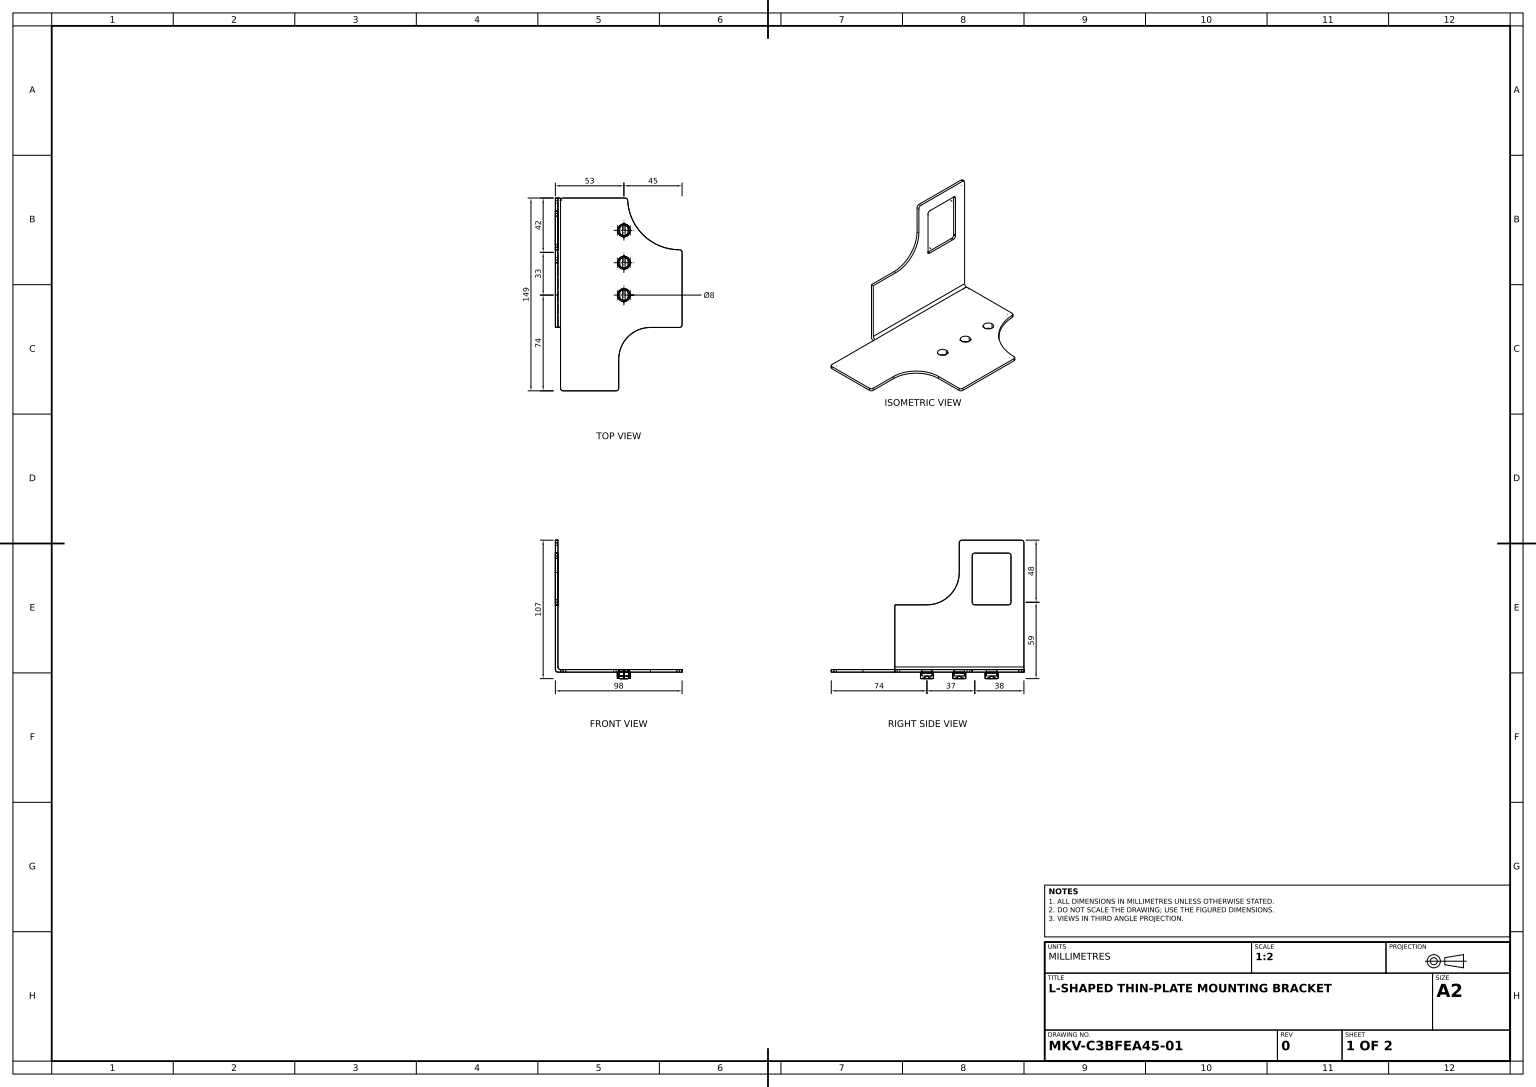
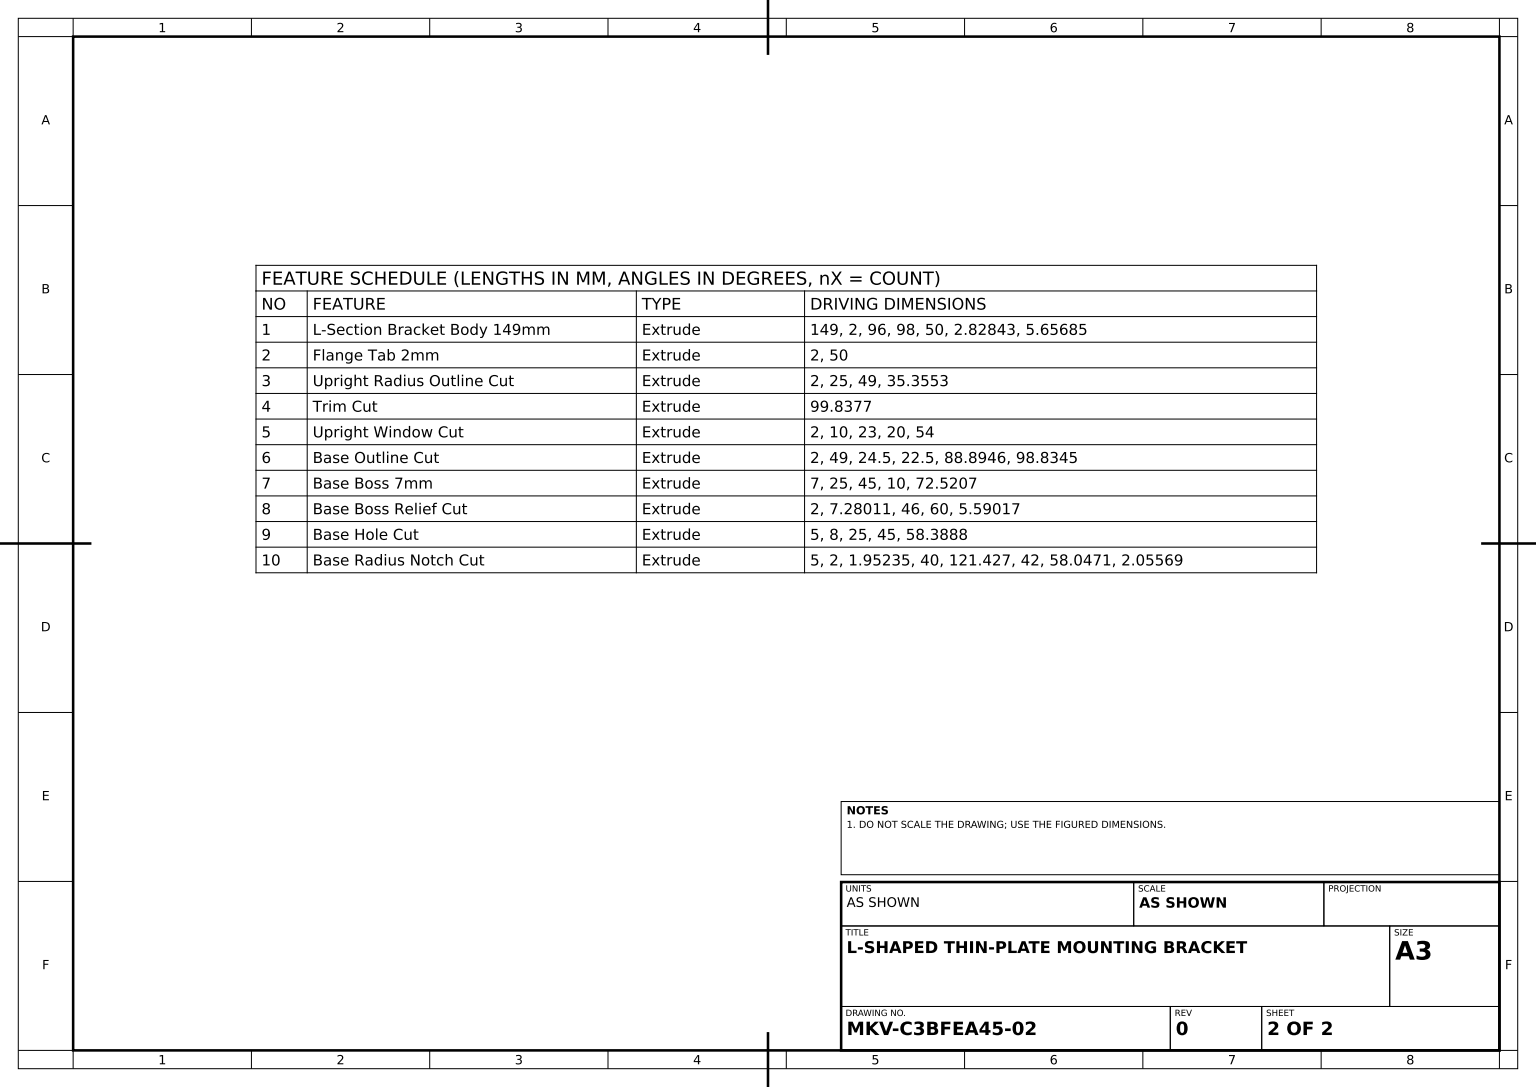
from build123d import *

# Parameters (mm, degrees)
L_SECTION_BRACKET_BODY_149MM_DEPTH = 74.5
FLANGE_TAB_SKETCH_W                = 149
FLANGE_TAB_SKETCH_H                = 50
FLANGE_TAB_2MM_DEPTH               = 2
UPRIGHT_RADIUS_OUTLINE_CUT_DEPTH   = 2
TRIM_CUT_DEPTH                     = 159.600914247
TRIM_CUT_DEPTH_BACK                = 159.600914247
TRIM_CUT_SKETCH_W                  = 4
TRIM_CUT_SKETCH_H                  = 49.162283459
UPRIGHT_WINDOW_CUT_DEPTH           = 2
BASE_OUTLINE_CUT_DEPTH             = 2
BASE_BOSS_SKETCH_R                 = 5
BASE_BOSS_7MM_DEPTH                = 7
BASE_BOSS_RELIEF_CUT_DEPTH         = 160.869478013
BASE_BOSS_RELIEF_CUT_DEPTH_BACK    = 160.869478013
BASE_HOLE_SKETCH_R                 = 4
BASE_HOLE_CUT_DEPTH                = 5
BASE_RADIUS_NOTCH_CUT_DEPTH        = 5


with BuildPart() as part:
    # L-Section Profile Sketch → L-Section Bracket Body 149mm (new, symmetric)
    with BuildSketch(Plane.XY):
        with BuildLine():
            Line((2, 0), (98, 0))
            Line((98, 0), (98, 2))
            Line((98, 2), (4, 2))
            ThreePointArc((4, 2), (2.585786438, 2.585786438), (2, 4))
            Line((2, 4), (2, 52))
            Line((2, 52), (0, 52))
            Line((0, 52), (0, 2))
            ThreePointArc((0, 2), (0.585786438, 0.585786438), (2, 0))
        make_face()
    extrude(amount=L_SECTION_BRACKET_BODY_149MM_DEPTH, both=True)

    # Flange Tab Sketch → Flange Tab 2mm (add)
    with BuildSketch(Plane(origin=(2, 0, 0), x_dir=(0, 0, -1), z_dir=(1, 0, 0))):
        with Locations((0, 77)):
            Rectangle(FLANGE_TAB_SKETCH_W, FLANGE_TAB_SKETCH_H)
    extrude(amount=-FLANGE_TAB_2MM_DEPTH)

    # Upright Radius Outline Sketch → Upright Radius Outline Cut (cut)
    with BuildSketch(Plane(origin=(2, 0, 0), x_dir=(0, 0, -1), z_dir=(1, 0, 0))):
        with BuildLine():
            Line((24.5, 102), (-74.5, 102))
            Line((-74.5, 102), (-74.5, 4))
            Line((-74.5, 4), (-25.5, 4))
            Line((-25.5, 4), (-25.5, 52))
            Line((-25.5, 52), (-0.5, 52))
            ThreePointArc((-0.5, 52), (17.17766953, 59.32233047), (24.5, 77))
            Line((24.5, 77), (24.5, 102))
        make_face()
    extrude(amount=-UPRIGHT_RADIUS_OUTLINE_CUT_DEPTH, mode=Mode.SUBTRACT)

    # Trim Cut Sketch → Trim Cut (cut, two sides: drawn at the far end of the back side and taken through both)
    with BuildSketch(Plane(origin=(0, 2, 0), x_dir=(1, 0, 0), z_dir=(0, 1, 0)).offset(-TRIM_CUT_DEPTH_BACK)):
        with Locations((2, -49.918858271)):
            Rectangle(TRIM_CUT_SKETCH_W, TRIM_CUT_SKETCH_H)
    extrude(amount=TRIM_CUT_DEPTH + TRIM_CUT_DEPTH_BACK, mode=Mode.SUBTRACT)

    # Upright Window Sketch → Upright Window Cut (cut)
    with BuildSketch(Plane(origin=(2, 0, 0), x_dir=(0, 0, -1), z_dir=(1, 0, 0))):
        with BuildLine():
            ThreePointArc((24.5, 100), (25.085786438, 101.414213562), (26.5, 102))
            Line((26.5, 102), (24.5, 102))
            Line((24.5, 102), (24.5, 100))
        make_face()
        with BuildLine():
            Line((74.5, 100), (74.5, 102))
            Line((74.5, 102), (72.5, 102))
            ThreePointArc((72.5, 102), (73.914213562, 101.414213562), (74.5, 100))
        make_face()
        with BuildLine():
            ThreePointArc((36.5, 52), (35.085786438, 52.585786438), (34.5, 54))
            Line((34.5, 54), (34.5, 90))
            ThreePointArc((34.5, 90), (35.085786438, 91.414213562), (36.5, 92))
            Line((36.5, 92), (62.5, 92))
            ThreePointArc((62.5, 92), (63.914213562, 91.414213562), (64.5, 90))
            Line((64.5, 90), (64.5, 54))
            ThreePointArc((64.5, 54), (63.914213562, 52.585786438), (62.5, 52))
            Line((62.5, 52), (36.5, 52))
        make_face()
    extrude(amount=-UPRIGHT_WINDOW_CUT_DEPTH, mode=Mode.SUBTRACT)

    # Base Outline Sketch → Base Outline Cut (cut)
    with BuildSketch(Plane(origin=(0, 2, 0), x_dir=(1, 0, 0), z_dir=(0, 1, 0))):
        with BuildLine():
            Line((6, 74.5), (4, 74.5))
            Line((4, 74.5), (4, 72.5))
            ThreePointArc((4, 72.5), (4.585786438, 73.914213562), (6, 74.5))
        make_face()
        with BuildLine():
            Line((98, -74.5), (98, -23.5))
            ThreePointArc((98, -23.5), (97.414213562, -24.914213562), (96, -25.5))
            Line((96, -25.5), (73.5, -25.5))
            ThreePointArc((73.5, -25.5), (56.175883861, -32.675883861), (49, -50))
            Line((49, -50), (49, -72.5))
            ThreePointArc((49, -72.5), (48.414213562, -73.914213562), (47, -74.5))
            Line((47, -74.5), (98, -74.5))
        make_face()
        with BuildLine():
            ThreePointArc((6, -74.5), (4.585786438, -73.914213562), (4, -72.5))
            Line((4, -72.5), (4, -74.5))
            Line((4, -74.5), (6, -74.5))
        make_face()
    extrude(amount=-BASE_OUTLINE_CUT_DEPTH, mode=Mode.SUBTRACT)

    # Base Boss Sketch → Base Boss 7mm (add)
    with BuildSketch(Plane(origin=(0, 2, 0), x_dir=(1, 0, 0), z_dir=(0, 1, 0))):
        with Locations(Location((53, 24.5, 0), (0, 0, 270))):
            Circle(BASE_BOSS_SKETCH_R)
        with Locations(Location((53, 49.5, 0), (0, 0, 270))):
            Circle(BASE_BOSS_SKETCH_R)
        with Locations(Location((53, -0.5, 0), (0, 0, 270))):
            Circle(BASE_BOSS_SKETCH_R)
    extrude(amount=-BASE_BOSS_7MM_DEPTH)

    # Base Boss Relief Sketch → Base Boss Relief Cut (cut, two sides: drawn at the far end of the back side and taken through both)
    with BuildSketch(Plane.XY.offset(-BASE_BOSS_RELIEF_CUT_DEPTH_BACK)):
        with BuildLine():
            ThreePointArc((48, -3), (48.585786438, -4.414213562), (50, -5))
            Line((50, -5), (48, -5))
            Line((48, -5), (48, -3))
        make_face()
        with BuildLine():
            Line((58, -3), (58, -5))
            Line((58, -5), (56, -5))
            ThreePointArc((56, -5), (57.414213562, -4.414213562), (58, -3))
        make_face()
    extrude(amount=BASE_BOSS_RELIEF_CUT_DEPTH + BASE_BOSS_RELIEF_CUT_DEPTH_BACK, mode=Mode.SUBTRACT)

    # Base Hole Sketch → Base Hole Cut (cut)
    with BuildSketch(Plane(origin=(0, 2, 0), x_dir=(1, 0, 0), z_dir=(0, 1, 0))):
        with Locations(Location((53, 24.5, 0), (0, 0, 270))):
            Circle(BASE_HOLE_SKETCH_R)
        with Locations(Location((53, 49.5, 0), (0, 0, 270))):
            Circle(BASE_HOLE_SKETCH_R)
        with Locations(Location((53, -0.5, 0), (0, 0, 90))):
            Circle(BASE_HOLE_SKETCH_R)
    extrude(amount=-BASE_HOLE_CUT_DEPTH, mode=Mode.SUBTRACT)

    # Base Radius Notch Sketch → Base Radius Notch Cut (cut)
    with BuildSketch(Plane(origin=(0, 2, 0), x_dir=(1, 0, 0), z_dir=(0, 1, 0))):
        with BuildLine():
            Line((55.887172383, 74.5), (53.934818456, 74.5))
            ThreePointArc((53.934818456, 74.5), (55.314949575, 73.947493729), (55.932549596, 72.595238095))
            ThreePointArc((55.932549596, 72.595238095), (68.323460008, 45.51307605), (95.994627256, 34.500144332))
            ThreePointArc((95.994627256, 34.500144332), (97.412312733, 33.916263389), (98, 32.500151549))
            Line((98, 32.500151549), (98, 34.555839482))
            Line((98, 34.555839482), (98, 74.5))
            Line((98, 74.5), (55.887172383, 74.5))
        make_face()
    extrude(amount=-BASE_RADIUS_NOTCH_CUT_DEPTH, mode=Mode.SUBTRACT)


solid = part.part
